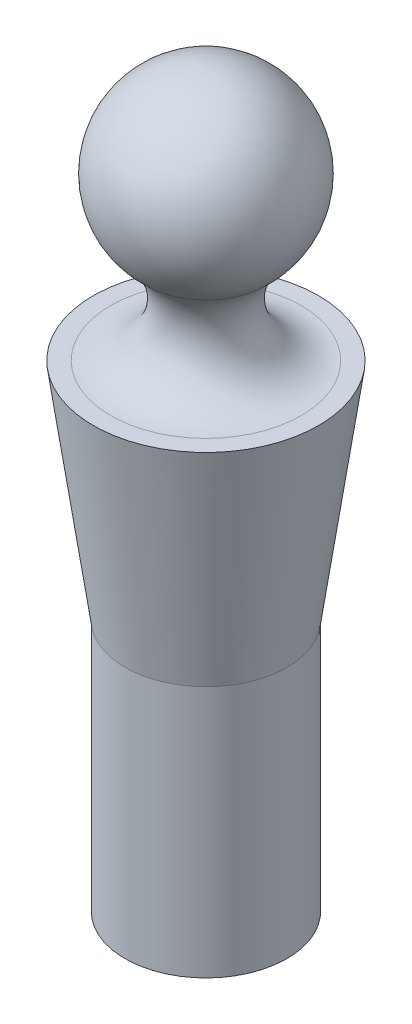
SolidWorks part; units mm, degrees
material "Plain Carbon Steel"
ref_plane "Front Plane" through (0, 0, 0) normal (0, 0, 1) x (1, 0, 0)
ref_plane "Top Plane" through (0, 0, 0) normal (0, 1, 0) x (1, 0, 0)
ref_plane "Right Plane" through (0, 0, 0) normal (1, 0, 0) x (0, 0, -1)
sketch "Pin Profile Sketch" plane through (0, 0, 0) normal (0, 0, 1) x (1, 0, 0)
  line L0 (0, 0) -> (0, 71.2709) construction
  line L2 (9, 4.6611) -> (12.5, 29.6611)
  line L3 (12.5, 29.6611) -> (10.583, 29.6611)
  line L4 (0, 29.6611) -> (0, 0)
  line L5 (9, 4.6611) -> (9, -23.3389)
  line L6 (9, -23.3389) -> (0, -23.3389)
  line L7 (0, -23.3389) -> (0, 0)
  line L8 (0, 57.6611) -> (0, 29.6611)
  arc A0 (6.6144, 40.1611) -> (0, 57.6611) centre (0, 47.6611) ccw
  arc A1 (6.6144, 40.1611) -> (10.583, 29.6611) centre (10.583, 35.6611) ccw
  dimension "D6" = 20
  dimension "D7" = 6
  dimension "D1" = 12.5
  dimension "D2" = 9
  dimension "D3" = 28
  dimension "D4" = 25
  dimension "D5" = 23.3389
  dimension "D8" = 18
revolve "Pin Body Revolve" add sketch "Pin Profile Sketch" angle 360 about L0
